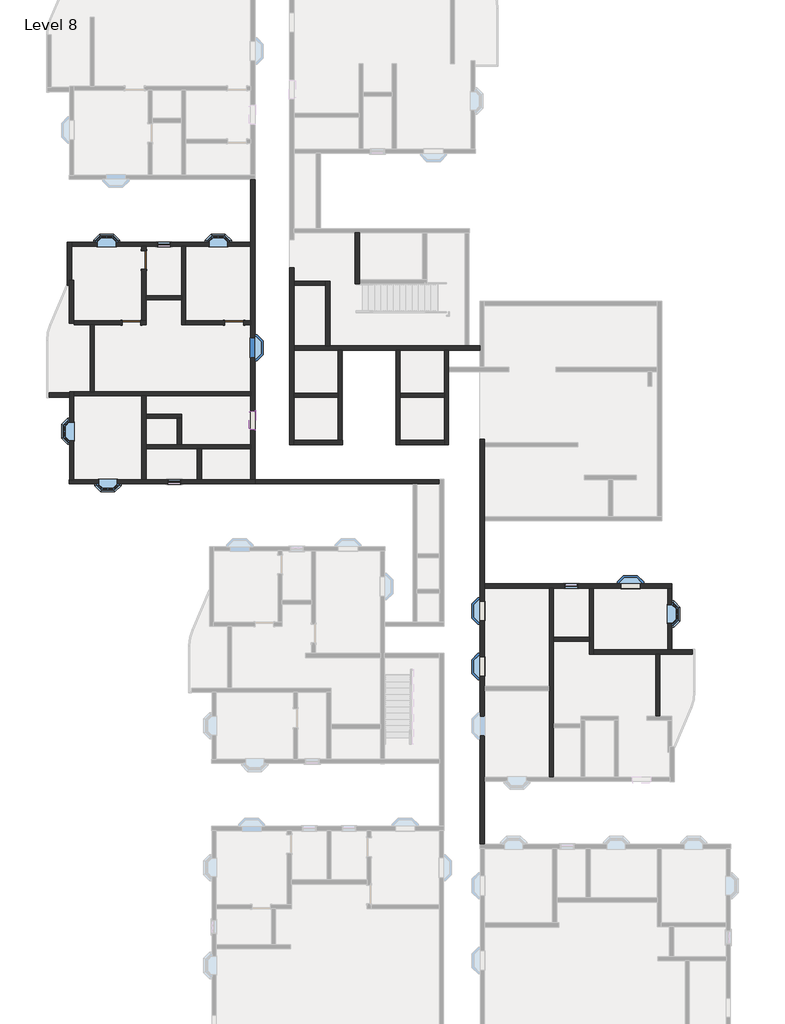
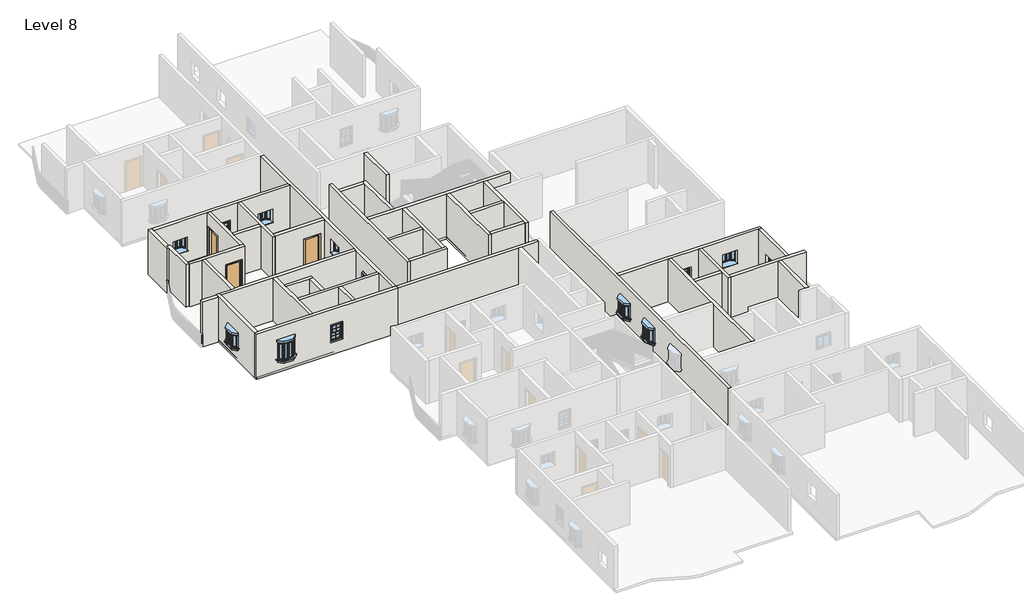
# One storey, part 3 of 14: 40 walls, 13 windows, 3 doors.
"""IFC4 building model written with IfcOpenShell, lengths in millimetres."""

from ifc_helpers import new_model, si_unit, frame, origin, place, context, project, spatial, polyline, outline, extrude, faceted_brep, transform, mapped, element, save
from components import door_54dd4da4, window_910x1210mm_154f9356, window_910x910mm_67ef725a, window_8debb0fa, windows_sgl_w_glazing_bars_910x910mm_256712d0

model = new_model("IFC4")

# Units and contexts
model_context = context("Model", 3, world=origin())
ifc_project = project(units=[si_unit("LENGTHUNIT", "METRE", prefix="MILLI")], contexts=[model_context])

# Site, building, storey
site = spatial("IfcSite", under=ifc_project)
building = spatial("IfcBuilding", under=site)
storey = spatial("IfcBuildingStorey", under=building, Name="Level 8", Elevation=21336.0)

# Doors
placement = place(None, origin())
door_shape = door_54dd4da4(model_context)
element("IfcDoor", 1, ObjectType="Single-Flush : 36\" x 84\"", at=placement, inside=storey, context=model_context, shape_type="MappedRepresentation", body=[
    mapped(door_shape, transform((-11210.3891351, 10605.7083494, 21336.0), x_axis=(1.0, 0.0, 0.0), y_axis=(0.0, 1.0, 0.0), z_axis=(0.0, 0.0, 1.0))),
])
element("IfcDoor", 2, ObjectType="Single-Flush : 36\" x 84\"", at=placement, inside=storey, context=model_context, shape_type="MappedRepresentation", body=[
    mapped(door_shape, transform((-15610.9391351, 13672.7583494, 21336.0), x_axis=(0.0, -1.0, 0.0), y_axis=(1.0, 0.0, 0.0), z_axis=(0.0, 0.0, 1.0))),
])
element("IfcDoor", 3, ObjectType="Single-Flush : 36\" x 84\"", at=placement, inside=storey, context=model_context, shape_type="MappedRepresentation", body=[
    mapped(door_shape, transform((-16220.5391351, 10605.7083494, 21336.0), x_axis=(1.0, 0.0, 0.0), y_axis=(0.0, 1.0, 0.0), z_axis=(0.0, 0.0, 1.0))),
])

# Walls
element("IfcWall", 4, ObjectType="4.5\" p", at=placement, inside=storey, context=model_context, shape_type="Brep", body=[
    faceted_brep([(-15509.3391351, 4456.3873146, 21336.0), (-13007.4391351, 4456.3873146, 21336.0), (-12804.2391351, 4456.3873146, 21336.0), (-10397.5891351, 4456.3873146, 21336.0), (-10397.5891351, 4456.3873146, 24384.0), (-12804.2391351, 4456.3873146, 24384.0), (-13007.4391351, 4456.3873146, 24384.0), (-15509.3391351, 4456.3873146, 24384.0), (-15509.3391351, 4659.5873146, 21336.0), (-15509.3391351, 4659.5873146, 24384.0), (-13985.3391351, 4659.5873146, 24384.0), (-13782.1391351, 4659.5873146, 24384.0), (-10397.5891351, 4659.5873146, 24384.0), (-10397.5891351, 4659.5873146, 21336.0), (-13782.1391351, 4659.5873146, 21336.0), (-13985.3391351, 4659.5873146, 21336.0)], [[[0, 1, 2, 3, 4, 5, 6, 7]], [[8, 9, 10, 11, 12, 13, 14, 15]], [[3, 2, 1, 0, 8, 15, 14, 13]], [[7, 6, 5, 4, 12, 11, 10, 9]], [[4, 3, 13, 12]], [[0, 7, 9, 8]]]),
])
element("IfcWall", 5, ObjectType="4.5\" p", at=placement, inside=storey, context=model_context, shape_type="SweptSolid", body=[
    extrude(outline(polyline([(-13007.4391351, 2953.9583494), (-13007.4391351, 4456.3873146), (-12804.2391351, 4456.3873146), (-12804.2391351, 2953.9583494), (-13007.4391351, 2953.9583494)])), frame((0.0, 0.0, 21336.0), z_axis=(0.0, 0.0, 1.0), x_axis=(1.0, 0.0, 0.0)), (0.0, 0.0, 1.0), 3048.0),
])
element("IfcWall", 6, ObjectType="4.5\" p", at=placement, inside=storey, context=model_context, shape_type="Brep", body=[
    faceted_brep([(-15509.3391351, 5953.2975261, 21336.0), (-13985.3391351, 5953.2975261, 21336.0), (-13782.1391351, 5953.2975261, 21336.0), (-13782.1391351, 5953.2975261, 24384.0), (-13985.3391351, 5953.2975261, 24384.0), (-15509.3391351, 5953.2975261, 24384.0), (-15509.3391351, 6156.4975261, 21336.0), (-15509.3391351, 6156.4975261, 24384.0), (-13782.1391351, 6156.4975261, 24384.0), (-13782.1391351, 6156.4975261, 21336.0)], [[[0, 1, 2, 3, 4, 5]], [[6, 7, 8, 9]], [[2, 1, 0, 6, 9]], [[5, 4, 3, 8, 7]], [[0, 5, 7, 6]], [[3, 2, 9, 8]]]),
])
element("IfcWall", 7, ObjectType="4.5\" p", at=placement, inside=storey, context=model_context, shape_type="SweptSolid", body=[
    extrude(outline(polyline([(-13985.3391351, 4659.5873146), (-13985.3391351, 5953.2975261), (-13782.1391351, 5953.2975261), (-13782.1391351, 4659.5873146), (-13985.3391351, 4659.5873146)])), frame((0.0, 0.0, 21336.0), z_axis=(0.0, 0.0, 1.0), x_axis=(1.0, 0.0, 0.0)), (0.0, 0.0, 1.0), 3048.0),
])
element("IfcWall", 8, ObjectType="4.5\" p", at=placement, inside=storey, context=model_context, shape_type="Brep", body=[
    faceted_brep([(-15712.5391351, 13215.5583494, 23469.6), (-15712.5391351, 13215.5583494, 21336.0), (-15712.5391351, 10707.3083494, 21336.0), (-15712.5391351, 10707.3083494, 24384.0), (-15712.5391351, 14333.1583494, 24384.0), (-15712.5391351, 14333.1583494, 21336.0), (-15712.5391351, 14129.9583494, 21336.0), (-15712.5391351, 14129.9583494, 23469.6), (-15509.3391351, 10707.3083494, 21336.0), (-15509.3391351, 11723.3083494, 21336.0), (-15509.3391351, 11926.5083494, 21336.0), (-15509.3391351, 13215.5583494, 21336.0), (-15509.3391351, 13215.5583494, 23469.6), (-15509.3391351, 14129.9583494, 23469.6), (-15509.3391351, 14129.9583494, 21336.0), (-15509.3391351, 14333.1583494, 21336.0), (-15509.3391351, 14333.1583494, 24384.0), (-15509.3391351, 11926.5083494, 24384.0), (-15509.3391351, 11723.3083494, 24384.0), (-15509.3391351, 10707.3083494, 24384.0)], [[[0, 1, 2, 3, 4, 5, 6, 7]], [[8, 9, 10, 11, 12, 13, 14, 15, 16, 17, 18, 19]], [[6, 5, 15, 14]], [[2, 1, 11, 10, 9, 8]], [[4, 3, 19, 18, 17, 16]], [[3, 2, 8, 19]], [[5, 4, 16, 15]], [[12, 11, 1, 0]], [[13, 12, 0, 7]], [[14, 13, 7, 6]]]),
])
element("IfcWall", 9, ObjectType="4.5\" p", at=placement, inside=storey, context=model_context, shape_type="Brep", body=[
    faceted_brep([(-13769.4391351, 14333.1583494, 21336.0), (-13769.4391351, 11926.5083494, 21336.0), (-13769.4391351, 11723.3083494, 21336.0), (-13769.4391351, 10504.1083494, 21336.0), (-13769.4391351, 10504.1083494, 24384.0), (-13769.4391351, 11723.3083494, 24384.0), (-13769.4391351, 11926.5083494, 24384.0), (-13769.4391351, 14333.1583494, 24384.0), (-13566.2391351, 14333.1583494, 21336.0), (-13566.2391351, 14333.1583494, 24384.0), (-13566.2391351, 10707.3083494, 24384.0), (-13566.2391351, 10504.1083494, 24384.0), (-13566.2391351, 10504.1083494, 21336.0), (-13566.2391351, 10707.3083494, 21336.0)], [[[0, 1, 2, 3, 4, 5, 6, 7]], [[8, 9, 10, 11, 12, 13]], [[3, 2, 1, 0, 8, 13, 12]], [[7, 6, 5, 4, 11, 10, 9]], [[0, 7, 9, 8]], [[4, 3, 12, 11]]]),
])
element("IfcWall", 10, ObjectType="4.5\" p", at=placement, inside=storey, context=model_context, shape_type="SweptSolid", body=[
    extrude(outline(polyline([(23469.6, -10753.1891351), (21336.0, -10753.1891351), (21336.0, -10397.5891351), (24384.0, -10397.5891351), (24384.0, -13566.2391351), (21336.0, -13566.2391351), (21336.0, -11667.5891351), (23469.6, -11667.5891351), (23469.6, -10753.1891351)])), frame((0.0, 10504.1083494, 0.0), z_axis=(0.0, 1.0, 0.0), x_axis=(0.0, 0.0, 1.0)), (0.0, 0.0, 1.0), 203.2),
])
element("IfcWall", 11, ObjectType="4.5\" p", at=placement, inside=storey, context=model_context, shape_type="SweptSolid", body=[
    extrude(outline(polyline([(-13769.4391351, 11723.3083494), (-15509.3391351, 11723.3083494), (-15509.3391351, 11926.5083494), (-13769.4391351, 11926.5083494), (-13769.4391351, 11723.3083494)])), frame((0.0, 0.0, 21336.0), z_axis=(0.0, 0.0, 1.0), x_axis=(1.0, 0.0, 0.0)), (0.0, 0.0, 1.0), 3048.0),
])
element("IfcWall", 12, ObjectType="4.5\" p", at=placement, inside=storey, context=model_context, shape_type="SweptSolid", body=[
    extrude(outline(polyline([(-6739.9891351, 12429.8715905), (-8289.3891351, 12429.8715905), (-8289.3891351, 12633.0715905), (-6739.9891351, 12633.0715905), (-6739.9891351, 12429.8715905)])), frame((0.0, 0.0, 21336.0), z_axis=(0.0, 0.0, 1.0), x_axis=(1.0, 0.0, 0.0)), (0.0, 0.0, 1.0), 3048.0),
])
element("IfcWall", 13, ObjectType="4.5\" p", at=placement, inside=storey, context=model_context, shape_type="SweptSolid", body=[
    extrude(outline(polyline([(-6130.3891351, 6970.2449943), (-8289.3891351, 6970.2449943), (-8289.3891351, 7173.4449943), (-6130.3891351, 7173.4449943), (-6130.3891351, 6970.2449943)])), frame((0.0, 0.0, 21336.0), z_axis=(0.0, 0.0, 1.0), x_axis=(1.0, 0.0, 0.0)), (0.0, 0.0, 1.0), 3048.0),
])
element("IfcWall", 14, ObjectType="4.5\" p", at=placement, inside=storey, context=model_context, shape_type="SweptSolid", body=[
    extrude(outline(polyline([(-948.7891351, 6970.2449943), (-3107.7891351, 6970.2449943), (-3107.7891351, 7173.4449943), (-948.7891351, 7173.4449943), (-948.7891351, 6970.2449943)])), frame((0.0, 0.0, 21336.0), z_axis=(0.0, 0.0, 1.0), x_axis=(1.0, 0.0, 0.0)), (0.0, 0.0, 1.0), 3048.0),
])
element("IfcWall", 15, ObjectType="4.5\" p", at=placement, inside=storey, context=model_context, shape_type="Brep", body=[
    faceted_brep([(-5298.5391351, 14988.9215905, 21336.0), (-5298.5391351, 12506.0715905, 21336.0), (-5298.5391351, 12506.0715905, 24384.0), (-5298.5391351, 14988.9215905, 24384.0), (-5095.3391351, 14988.9215905, 21336.0), (-5095.3391351, 14988.9215905, 24384.0), (-5095.3391351, 12709.2715905, 24384.0), (-5095.3391351, 12506.0715905, 24384.0), (-5095.3391351, 12506.0715905, 21336.0), (-5095.3391351, 12709.2715905, 21336.0)], [[[0, 1, 2, 3]], [[4, 5, 6, 7, 8, 9]], [[1, 0, 4, 9, 8]], [[3, 2, 7, 6, 5]], [[0, 3, 5, 4]], [[2, 1, 8, 7]]]),
])
element("IfcWall", 16, ObjectType="4.5\" p", at=placement, inside=storey, context=model_context, shape_type="SweptSolid", body=[
    extrude(outline(polyline([(-948.7891351, 4665.1949943), (-3107.7891351, 4665.1949943), (-3107.7891351, 4868.3949943), (-948.7891351, 4868.3949943), (-948.7891351, 4665.1949943)])), frame((0.0, 0.0, 21336.0), z_axis=(0.0, 0.0, 1.0), x_axis=(1.0, 0.0, 0.0)), (0.0, 0.0, 1.0), 3048.0),
])
element("IfcWall", 17, ObjectType="4.5\" p", at=placement, inside=storey, context=model_context, shape_type="Brep", body=[
    faceted_brep([(4184.4880523, -2336.4042694, 21336.0), (4184.4880523, -7130.6542694, 21336.0), (4184.4880523, -7333.8542694, 21336.0), (4184.4880523, -11556.6042694, 21336.0), (4184.4880523, -11556.6042694, 24384.0), (4184.4880523, -7333.8542694, 24384.0), (4184.4880523, -7130.6542694, 24384.0), (4184.4880523, -2336.4042694, 24384.0), (4387.6880523, -2336.4042694, 21336.0), (4387.6880523, -2336.4042694, 24384.0), (4387.6880523, -4736.7042694, 24384.0), (4387.6880523, -4939.9042694, 24384.0), (4387.6880523, -8959.4542694, 24384.0), (4387.6880523, -9162.6542694, 24384.0), (4387.6880523, -11556.6042694, 24384.0), (4387.6880523, -11556.6042694, 21336.0), (4387.6880523, -9162.6542694, 21336.0), (4387.6880523, -8959.4542694, 21336.0), (4387.6880523, -4939.9042694, 21336.0), (4387.6880523, -4736.7042694, 21336.0)], [[[0, 1, 2, 3, 4, 5, 6, 7]], [[8, 9, 10, 11, 12, 13, 14, 15, 16, 17, 18, 19]], [[3, 2, 1, 0, 8, 19, 18, 17, 16, 15]], [[7, 6, 5, 4, 14, 13, 12, 11, 10, 9]], [[4, 3, 15, 14]], [[0, 7, 9, 8]]]),
])
element("IfcWall", 18, ObjectType="4.5\" p", at=placement, inside=storey, context=model_context, shape_type="Brep", body=[
    faceted_brep([(803.8108649, 4915.2957306, 21336.0), (803.8108649, -14845.9042694, 21336.0), (803.8108649, -14845.9042694, 24384.0), (803.8108649, 4915.2957306, 24384.0), (803.8108649, -9516.0542694, 23446.0), (803.8108649, -9516.0542694, 22536.0), (803.8108649, -8606.0542694, 22536.0), (803.8108649, -8606.0542694, 23446.0), (803.8108649, -3909.0042694, 23446.0), (803.8108649, -3909.0042694, 22536.0), (803.8108649, -2999.0042694, 22536.0), (803.8108649, -2999.0042694, 23446.0), (803.8108649, -6620.4542694, 23446.0), (803.8108649, -6620.4542694, 22536.0), (803.8108649, -5710.4542694, 22536.0), (803.8108649, -5710.4542694, 23446.0), (1007.0108649, 4915.2957306, 21336.0), (1007.0108649, 4915.2957306, 24384.0), (1007.0108649, 4754.0949943, 24384.0), (1007.0108649, 4550.8949943, 24384.0), (1007.0108649, 1143.3957306, 24384.0), (1007.0108649, 940.1957306, 24384.0), (1007.0108649, -2133.2042694, 24384.0), (1007.0108649, -2336.4042694, 24384.0), (1007.0108649, -7130.6542694, 24384.0), (1007.0108649, -7333.8542694, 24384.0), (1007.0108649, -11556.6042694, 24384.0), (1007.0108649, -11759.8042694, 24384.0), (1007.0108649, -14845.9042694, 24384.0), (1007.0108649, -14845.9042694, 21336.0), (1007.0108649, -11759.8042694, 21336.0), (1007.0108649, -11556.6042694, 21336.0), (1007.0108649, -7333.8542694, 21336.0), (1007.0108649, -7130.6542694, 21336.0), (1007.0108649, -2336.4042694, 21336.0), (1007.0108649, -2133.2042694, 21336.0), (1007.0108649, 940.1957306, 21336.0), (1007.0108649, 1143.3957306, 21336.0), (1007.0108649, 4550.8949943, 21336.0), (1007.0108649, 4754.0949943, 21336.0), (1007.0108649, -9516.0542694, 23446.0), (1007.0108649, -8606.0542694, 23446.0), (1007.0108649, -8606.0542694, 22536.0), (1007.0108649, -9516.0542694, 22536.0), (1007.0108649, -3909.0042694, 23446.0), (1007.0108649, -2999.0042694, 23446.0), (1007.0108649, -2999.0042694, 22536.0), (1007.0108649, -3909.0042694, 22536.0), (1007.0108649, -6620.4542694, 23446.0), (1007.0108649, -5710.4542694, 23446.0), (1007.0108649, -5710.4542694, 22536.0), (1007.0108649, -6620.4542694, 22536.0)], [[[0, 1, 2, 3], [4, 5, 6, 7], [8, 9, 10, 11], [12, 13, 14, 15]], [[16, 17, 18, 19, 20, 21, 22, 23, 24, 25, 26, 27, 28, 29, 30, 31, 32, 33, 34, 35, 36, 37, 38, 39], [40, 41, 42, 43], [44, 45, 46, 47], [48, 49, 50, 51]], [[1, 0, 16, 39, 38, 37, 36, 35, 34, 33, 32, 31, 30, 29]], [[3, 2, 28, 27, 26, 25, 24, 23, 22, 21, 20, 19, 18, 17]], [[0, 3, 17, 16]], [[2, 1, 29, 28]], [[5, 4, 40, 43]], [[6, 5, 43, 42]], [[7, 6, 42, 41]], [[4, 7, 41, 40]], [[9, 8, 44, 47]], [[10, 9, 47, 46]], [[11, 10, 46, 45]], [[8, 11, 45, 44]], [[13, 12, 48, 51]], [[14, 13, 51, 50]], [[15, 14, 50, 49]], [[12, 15, 49, 48]]]),
])
element("IfcWall", 19, ObjectType="4.5\" p", at=placement, inside=storey, context=model_context, shape_type="SweptSolid", body=[
    extrude(outline(polyline([(6127.5880523, -4939.9042694), (4387.6880523, -4939.9042694), (4387.6880523, -4736.7042694), (6127.5880523, -4736.7042694), (6127.5880523, -4939.9042694)])), frame((0.0, 0.0, 21336.0), z_axis=(0.0, 0.0, 1.0), x_axis=(1.0, 0.0, 0.0)), (0.0, 0.0, 1.0), 3048.0),
])
element("IfcWall", 20, ObjectType="4.5\" p", at=placement, inside=storey, context=model_context, shape_type="Brep", body=[
    faceted_brep([(6127.5880523, -2336.4042694, 21336.0), (6127.5880523, -4736.7042694, 21336.0), (6127.5880523, -4939.9042694, 21336.0), (6127.5880523, -5555.8542694, 21336.0), (6127.5880523, -5555.8542694, 24384.0), (6127.5880523, -4939.9042694, 24384.0), (6127.5880523, -4736.7042694, 24384.0), (6127.5880523, -2336.4042694, 24384.0), (6330.7880523, -2336.4042694, 21336.0), (6330.7880523, -2336.4042694, 24384.0), (6330.7880523, -5352.6542694, 24384.0), (6330.7880523, -5555.8542694, 24384.0), (6330.7880523, -5555.8542694, 21336.0), (6330.7880523, -5352.6542694, 21336.0)], [[[0, 1, 2, 3, 4, 5, 6, 7]], [[8, 9, 10, 11, 12, 13]], [[3, 2, 1, 0, 8, 13, 12]], [[7, 6, 5, 4, 11, 10, 9]], [[0, 7, 9, 8]], [[4, 3, 12, 11]]]),
])
element("IfcWall", 21, ObjectType="4.5\" p", at=placement, inside=storey, context=model_context, shape_type="Brep", body=[
    faceted_brep([(6330.7880523, -5555.8542694, 21336.0), (9371.2322031, -5555.8542694, 21336.0), (9574.4322031, -5555.8542694, 21336.0), (11163.1380523, -5555.8542694, 21336.0), (11163.1380523, -5555.8542694, 24384.0), (9574.4322031, -5555.8542694, 24384.0), (9371.2322031, -5555.8542694, 24384.0), (6330.7880523, -5555.8542694, 24384.0), (6330.7880523, -5352.6542694, 21336.0), (6330.7880523, -5352.6542694, 24384.0), (9956.6380523, -5352.6542694, 24384.0), (10159.8380523, -5352.6542694, 24384.0), (11163.1380523, -5352.6542694, 24384.0), (11163.1380523, -5352.6542694, 21336.0), (10159.8380523, -5352.6542694, 21336.0), (9956.6380523, -5352.6542694, 21336.0)], [[[0, 1, 2, 3, 4, 5, 6, 7]], [[8, 9, 10, 11, 12, 13, 14, 15]], [[3, 2, 1, 0, 8, 15, 14, 13]], [[4, 3, 13, 12]], [[7, 6, 5, 4, 12, 11, 10, 9]], [[0, 7, 9, 8]]]),
])
element("IfcWall", 22, ObjectType="4.5\" p", at=placement, inside=storey, context=model_context, shape_type="SweptSolid", body=[
    extrude(outline(polyline([(9371.2322031, -8578.4542694), (9371.2322031, -5555.8542694), (9574.4322031, -5555.8542694), (9574.4322031, -8578.4542694), (9371.2322031, -8578.4542694)])), frame((0.0, 0.0, 21336.0), z_axis=(0.0, 0.0, 1.0), x_axis=(1.0, 0.0, 0.0)), (0.0, 0.0, 1.0), 3048.0),
])
element("IfcWall", 23, ObjectType="9\"", at=placement, inside=storey, context=model_context, shape_type="Brep", body=[
    faceted_brep([(-10181.6891351, 2953.9583494, 21336.0), (-10194.3891351, 2953.9583494, 21336.0), (-10397.5891351, 2953.9583494, 21336.0), (-12804.2391351, 2953.9583494, 21336.0), (-13007.4391351, 2953.9583494, 21336.0), (-15509.3391351, 2953.9583494, 21336.0), (-15712.5391351, 2953.9583494, 21336.0), (-19033.5891351, 2953.9583494, 21336.0), (-19236.7891351, 2953.9583494, 21336.0), (-19249.4891351, 2953.9583494, 21336.0), (-19249.4891351, 2953.9583494, 24384.0), (-19236.7891351, 2953.9583494, 24384.0), (-19033.5891351, 2953.9583494, 24384.0), (-15712.5391351, 2953.9583494, 24384.0), (-15509.3391351, 2953.9583494, 24384.0), (-13007.4391351, 2953.9583494, 24384.0), (-12804.2391351, 2953.9583494, 24384.0), (-10397.5891351, 2953.9583494, 24384.0), (-10194.3891351, 2953.9583494, 24384.0), (-10181.6891351, 2953.9583494, 24384.0), (-13794.8391351, 2953.9583494, 23317.2), (-14455.2391351, 2953.9583494, 23317.2), (-14455.2391351, 2953.9583494, 22250.4), (-13794.8391351, 2953.9583494, 22250.4), (-16918.0641351, 2953.9583494, 23446.0), (-17828.0641351, 2953.9583494, 23446.0), (-17828.0641351, 2953.9583494, 22236.0), (-16918.0641351, 2953.9583494, 22236.0), (-10181.6891351, 2750.7583494, 21336.0), (-10181.6891351, 2750.7583494, 24384.0), (-19249.4891351, 2750.7583494, 24384.0), (-19249.4891351, 2750.7583494, 21336.0), (-13794.8391351, 2750.7583494, 23317.2), (-13794.8391351, 2750.7583494, 22250.4), (-14455.2391351, 2750.7583494, 22250.4), (-14455.2391351, 2750.7583494, 23317.2), (-16918.0641351, 2750.7583494, 23446.0), (-16918.0641351, 2750.7583494, 22236.0), (-17828.0641351, 2750.7583494, 22236.0), (-17828.0641351, 2750.7583494, 23446.0)], [[[0, 1, 2, 3, 4, 5, 6, 7, 8, 9, 10, 11, 12, 13, 14, 15, 16, 17, 18, 19], [20, 21, 22, 23], [24, 25, 26, 27]], [[28, 29, 30, 31], [32, 33, 34, 35], [36, 37, 38, 39]], [[9, 8, 7, 6, 5, 4, 3, 2, 1, 0, 28, 31]], [[10, 9, 31, 30]], [[19, 18, 17, 16, 15, 14, 13, 12, 11, 10, 30, 29]], [[0, 19, 29, 28]], [[33, 32, 20, 23]], [[34, 33, 23, 22]], [[35, 34, 22, 21]], [[32, 35, 21, 20]], [[37, 36, 24, 27]], [[38, 37, 27, 26]], [[39, 38, 26, 25]], [[36, 39, 25, 24]]]),
])
element("IfcWall", 24, ObjectType="9\"", at=placement, inside=storey, context=model_context, shape_type="Brep", body=[
    faceted_brep([(-19033.5891351, 2953.9583494, 21336.0), (-19033.5891351, 7037.0083494, 21336.0), (-19033.5891351, 7240.2083494, 21336.0), (-19033.5891351, 7240.2083494, 24384.0), (-19033.5891351, 7037.0083494, 24384.0), (-19033.5891351, 2953.9583494, 24384.0), (-19033.5891351, 4854.8083494, 23160.4), (-19033.5891351, 5764.8083494, 23160.4), (-19033.5891351, 5764.8083494, 22250.4), (-19033.5891351, 4854.8083494, 22250.4), (-19236.7891351, 2953.9583494, 21336.0), (-19236.7891351, 2953.9583494, 24384.0), (-19236.7891351, 7240.2083494, 24384.0), (-19236.7891351, 7240.2083494, 21336.0), (-19236.7891351, 4854.8083494, 23160.4), (-19236.7891351, 4854.8083494, 22250.4), (-19236.7891351, 5764.8083494, 22250.4), (-19236.7891351, 5764.8083494, 23160.4)], [[[0, 1, 2, 3, 4, 5], [6, 7, 8, 9]], [[10, 11, 12, 13], [14, 15, 16, 17]], [[2, 1, 0, 10, 13]], [[5, 4, 3, 12, 11]], [[0, 5, 11, 10]], [[3, 2, 13, 12]], [[15, 14, 6, 9]], [[16, 15, 9, 8]], [[17, 16, 8, 7]], [[14, 17, 7, 6]]]),
])
element("IfcWall", 25, ObjectType="9\"", at=placement, inside=storey, context=model_context, shape_type="Brep", body=[
    faceted_brep([(-10194.3891351, 2953.9583494, 21336.0), (-10194.3891351, 17597.0583494, 21336.0), (-10194.3891351, 17597.0583494, 24384.0), (-10194.3891351, 2953.9583494, 24384.0), (-10194.3891351, 9841.5083494, 23446.0), (-10194.3891351, 9841.5083494, 22536.0), (-10194.3891351, 8931.5083494, 22536.0), (-10194.3891351, 8931.5083494, 23446.0), (-10194.3891351, 5393.297832, 23446.0), (-10194.3891351, 6303.297832, 23446.0), (-10194.3891351, 6303.297832, 22536.0), (-10194.3891351, 5393.297832, 22536.0), (-10397.5891351, 2953.9583494, 21336.0), (-10397.5891351, 2953.9583494, 24384.0), (-10397.5891351, 4456.3873146, 24384.0), (-10397.5891351, 4659.5873146, 24384.0), (-10397.5891351, 7037.0083494, 24384.0), (-10397.5891351, 7240.2083494, 24384.0), (-10397.5891351, 10504.1083494, 24384.0), (-10397.5891351, 10707.3083494, 24384.0), (-10397.5891351, 14333.1583494, 24384.0), (-10397.5891351, 14536.3583494, 24384.0), (-10397.5891351, 17597.0583494, 24384.0), (-10397.5891351, 17597.0583494, 21336.0), (-10397.5891351, 14536.3583494, 21336.0), (-10397.5891351, 14333.1583494, 21336.0), (-10397.5891351, 10707.3083494, 21336.0), (-10397.5891351, 10504.1083494, 21336.0), (-10397.5891351, 7240.2083494, 21336.0), (-10397.5891351, 7037.0083494, 21336.0), (-10397.5891351, 4659.5873146, 21336.0), (-10397.5891351, 4456.3873146, 21336.0), (-10397.5891351, 9841.5083494, 23446.0), (-10397.5891351, 8931.5083494, 23446.0), (-10397.5891351, 8931.5083494, 22536.0), (-10397.5891351, 9841.5083494, 22536.0), (-10397.5891351, 5393.297832, 23446.0), (-10397.5891351, 5393.297832, 22536.0), (-10397.5891351, 6303.297832, 22536.0), (-10397.5891351, 6303.297832, 23446.0)], [[[0, 1, 2, 3], [4, 5, 6, 7], [8, 9, 10, 11]], [[12, 13, 14, 15, 16, 17, 18, 19, 20, 21, 22, 23, 24, 25, 26, 27, 28, 29, 30, 31], [32, 33, 34, 35], [36, 37, 38, 39]], [[1, 0, 12, 31, 30, 29, 28, 27, 26, 25, 24, 23]], [[2, 1, 23, 22]], [[3, 2, 22, 21, 20, 19, 18, 17, 16, 15, 14, 13]], [[0, 3, 13, 12]], [[5, 4, 32, 35]], [[6, 5, 35, 34]], [[7, 6, 34, 33]], [[4, 7, 33, 32]], [[37, 36, 8, 11]], [[38, 37, 11, 10]], [[39, 38, 10, 9]], [[36, 39, 9, 8]]]),
])
element("IfcWall", 26, ObjectType="9\"", at=placement, inside=storey, context=model_context, shape_type="SweptSolid", body=[
    extrude(outline(polyline([(-19249.4891351, 6979.8583494), (-20240.0891351, 6979.8583494), (-20240.0891351, 7183.0583494), (-19249.4891351, 7183.0583494), (-19249.4891351, 6979.8583494)])), frame((0.0, 0.0, 21336.0), z_axis=(0.0, 0.0, 1.0), x_axis=(1.0, 0.0, 0.0)), (0.0, 0.0, 1.0), 3048.0),
])
element("IfcWall", 27, ObjectType="9\"", at=placement, inside=storey, context=model_context, shape_type="Brep", body=[
    faceted_brep([(-19147.8891351, 12435.1858981, 21336.0), (-19147.8891351, 14333.1583494, 21336.0), (-19147.8891351, 14536.3583494, 21336.0), (-19147.8891351, 14549.0583494, 21336.0), (-19147.8891351, 14549.0583494, 24384.0), (-19147.8891351, 14536.3583494, 24384.0), (-19147.8891351, 14333.1583494, 24384.0), (-19147.8891351, 12435.1858981, 24384.0), (-19351.0891351, 12435.1858981, 21336.0), (-19351.0891351, 12435.1858981, 24384.0), (-19351.0891351, 14549.0583494, 24384.0), (-19351.0891351, 14549.0583494, 21336.0)], [[[0, 1, 2, 3, 4, 5, 6, 7]], [[8, 9, 10, 11]], [[3, 2, 1, 0, 8, 11]], [[4, 3, 11, 10]], [[7, 6, 5, 4, 10, 9]], [[0, 7, 9, 8]]]),
])
element("IfcWall", 28, ObjectType="9\"", at=placement, inside=storey, context=model_context, shape_type="Brep", body=[
    faceted_brep([(-19147.8891351, 14333.1583494, 21336.0), (-15712.5391351, 14333.1583494, 21336.0), (-15509.3391351, 14333.1583494, 21336.0), (-13769.4391351, 14333.1583494, 21336.0), (-13566.2391351, 14333.1583494, 21336.0), (-10397.5891351, 14333.1583494, 21336.0), (-10397.5891351, 14333.1583494, 24384.0), (-13566.2391351, 14333.1583494, 24384.0), (-13769.4391351, 14333.1583494, 24384.0), (-15509.3391351, 14333.1583494, 24384.0), (-15712.5391351, 14333.1583494, 24384.0), (-19147.8891351, 14333.1583494, 24384.0), (-17885.2141351, 14333.1583494, 23160.4), (-16975.2141351, 14333.1583494, 23160.4), (-16975.2141351, 14333.1583494, 22250.4), (-17885.2141351, 14333.1583494, 22250.4), (-12436.9141351, 14333.1583494, 23160.4), (-11526.9141351, 14333.1583494, 23160.4), (-11526.9141351, 14333.1583494, 22250.4), (-12436.9141351, 14333.1583494, 22250.4), (-14309.1891351, 14333.1583494, 23317.2), (-14309.1891351, 14333.1583494, 22250.4), (-14969.5891351, 14333.1583494, 22250.4), (-14969.5891351, 14333.1583494, 23317.2), (-19147.8891351, 14536.3583494, 21336.0), (-19147.8891351, 14536.3583494, 24384.0), (-10397.5891351, 14536.3583494, 24384.0), (-10397.5891351, 14536.3583494, 21336.0), (-17885.2141351, 14536.3583494, 23160.4), (-17885.2141351, 14536.3583494, 22250.4), (-16975.2141351, 14536.3583494, 22250.4), (-16975.2141351, 14536.3583494, 23160.4), (-12436.9141351, 14536.3583494, 23160.4), (-12436.9141351, 14536.3583494, 22250.4), (-11526.9141351, 14536.3583494, 22250.4), (-11526.9141351, 14536.3583494, 23160.4), (-14309.1891351, 14536.3583494, 23317.2), (-14969.5891351, 14536.3583494, 23317.2), (-14969.5891351, 14536.3583494, 22250.4), (-14309.1891351, 14536.3583494, 22250.4)], [[[0, 1, 2, 3, 4, 5, 6, 7, 8, 9, 10, 11], [12, 13, 14, 15], [16, 17, 18, 19], [20, 21, 22, 23]], [[24, 25, 26, 27], [28, 29, 30, 31], [32, 33, 34, 35], [36, 37, 38, 39]], [[5, 4, 3, 2, 1, 0, 24, 27]], [[11, 10, 9, 8, 7, 6, 26, 25]], [[6, 5, 27, 26]], [[0, 11, 25, 24]], [[29, 28, 12, 15]], [[30, 29, 15, 14]], [[31, 30, 14, 13]], [[28, 31, 13, 12]], [[33, 32, 16, 19]], [[34, 33, 19, 18]], [[35, 34, 18, 17]], [[32, 35, 17, 16]], [[21, 20, 36, 39]], [[22, 21, 39, 38]], [[23, 22, 38, 37]], [[20, 23, 37, 36]]]),
])
element("IfcWall", 29, ObjectType="9\"", at=placement, inside=storey, context=model_context, shape_type="SweptSolid", body=[
    extrude(outline(polyline([(-19249.4891351, 10585.5474528), (-19249.4891351, 12672.4473407), (-19046.2891351, 12672.4473407), (-19046.2891351, 10585.5474528), (-19249.4891351, 10585.5474528)])), frame((0.0, 0.0, 21336.0), z_axis=(0.0, 0.0, 1.0), x_axis=(1.0, 0.0, 0.0)), (0.0, 0.0, 1.0), 3048.0),
])
element("IfcWall", 30, ObjectType="9\" w", at=placement, inside=storey, context=model_context, shape_type="Brep", body=[
    faceted_brep([(-1177.3891351, 2953.9583494, 21336.0), (-10181.6891351, 2953.9583494, 21336.0), (-10181.6891351, 2953.9583494, 24384.0), (-1177.3891351, 2953.9583494, 24384.0), (-1177.3891351, 2750.7583494, 21336.0), (-1177.3891351, 2750.7583494, 24384.0), (-2269.5891351, 2750.7583494, 24384.0), (-2472.7891351, 2750.7583494, 24384.0), (-10181.6891351, 2750.7583494, 24384.0), (-10181.6891351, 2750.7583494, 21336.0), (-2472.7891351, 2750.7583494, 21336.0), (-2269.5891351, 2750.7583494, 21336.0)], [[[0, 1, 2, 3]], [[4, 5, 6, 7, 8, 9, 10, 11]], [[1, 0, 4, 11, 10, 9]], [[2, 1, 9, 8]], [[3, 2, 8, 7, 6, 5]], [[0, 3, 5, 4]]]),
])
element("IfcWall", 31, ObjectType="9\" w", at=placement, inside=storey, context=model_context, shape_type="Brep", body=[
    faceted_brep([(-15763.3391351, 10504.1083494, 23469.6), (-15763.3391351, 10504.1083494, 21336.0), (-15509.3391351, 10504.1083494, 21336.0), (-15509.3391351, 10504.1083494, 24384.0), (-18042.9891351, 10504.1083494, 24384.0), (-18246.1891351, 10504.1083494, 24384.0), (-19027.2391351, 10504.1083494, 24384.0), (-19027.2391351, 10504.1083494, 21336.0), (-18246.1891351, 10504.1083494, 21336.0), (-18042.9891351, 10504.1083494, 21336.0), (-16677.7391351, 10504.1083494, 21336.0), (-16677.7391351, 10504.1083494, 23469.6), (-15509.3391351, 10707.3083494, 21336.0), (-15712.5391351, 10707.3083494, 21336.0), (-15763.3391351, 10707.3083494, 21336.0), (-15763.3391351, 10707.3083494, 23469.6), (-16677.7391351, 10707.3083494, 23469.6), (-16677.7391351, 10707.3083494, 21336.0), (-19027.2391351, 10707.3083494, 21336.0), (-19027.2391351, 10707.3083494, 24384.0), (-15712.5391351, 10707.3083494, 24384.0), (-15509.3391351, 10707.3083494, 24384.0)], [[[0, 1, 2, 3, 4, 5, 6, 7, 8, 9, 10, 11]], [[12, 13, 14, 15, 16, 17, 18, 19, 20, 21]], [[2, 1, 14, 13, 12]], [[10, 9, 8, 7, 18, 17]], [[6, 5, 4, 3, 21, 20, 19]], [[7, 6, 19, 18]], [[3, 2, 12, 21]], [[15, 14, 1, 0]], [[16, 15, 0, 11]], [[17, 16, 11, 10]]]),
])
element("IfcWall", 32, ObjectType="9\" w", at=placement, inside=storey, context=model_context, shape_type="SweptSolid", body=[
    extrude(outline(polyline([(-18246.1891351, 7240.2083494), (-18246.1891351, 10504.1083494), (-18042.9891351, 10504.1083494), (-18042.9891351, 7240.2083494), (-18246.1891351, 7240.2083494)])), frame((0.0, 0.0, 21336.0), z_axis=(0.0, 0.0, 1.0), x_axis=(1.0, 0.0, 0.0)), (0.0, 0.0, 1.0), 3048.0),
])
element("IfcWall", 33, ObjectType="9\" w", at=placement, inside=storey, context=model_context, shape_type="Brep", body=[
    faceted_brep([(-19033.5891351, 7037.0083494, 21336.0), (-15712.5391351, 7037.0083494, 21336.0), (-15509.3391351, 7037.0083494, 21336.0), (-10397.5891351, 7037.0083494, 21336.0), (-10397.5891351, 7037.0083494, 24384.0), (-15509.3391351, 7037.0083494, 24384.0), (-15712.5391351, 7037.0083494, 24384.0), (-19033.5891351, 7037.0083494, 24384.0), (-19033.5891351, 7240.2083494, 21336.0), (-19033.5891351, 7240.2083494, 24384.0), (-18246.1891351, 7240.2083494, 24384.0), (-18042.9891351, 7240.2083494, 24384.0), (-10397.5891351, 7240.2083494, 24384.0), (-10397.5891351, 7240.2083494, 21336.0), (-18042.9891351, 7240.2083494, 21336.0), (-18246.1891351, 7240.2083494, 21336.0)], [[[0, 1, 2, 3, 4, 5, 6, 7]], [[8, 9, 10, 11, 12, 13, 14, 15]], [[3, 2, 1, 0, 8, 15, 14, 13]], [[7, 6, 5, 4, 12, 11, 10, 9]], [[0, 7, 9, 8]], [[4, 3, 13, 12]]]),
])
element("IfcWall", 34, ObjectType="9\" w", at=placement, inside=storey, context=model_context, shape_type="Brep", body=[
    faceted_brep([(-15712.5391351, 7037.0083494, 21336.0), (-15712.5391351, 2953.9583494, 21336.0), (-15712.5391351, 2953.9583494, 24384.0), (-15712.5391351, 7037.0083494, 24384.0), (-15509.3391351, 7037.0083494, 21336.0), (-15509.3391351, 7037.0083494, 24384.0), (-15509.3391351, 6156.4975261, 24384.0), (-15509.3391351, 5953.2975261, 24384.0), (-15509.3391351, 4659.5873146, 24384.0), (-15509.3391351, 4456.3873146, 24384.0), (-15509.3391351, 2953.9583494, 24384.0), (-15509.3391351, 2953.9583494, 21336.0), (-15509.3391351, 4456.3873146, 21336.0), (-15509.3391351, 4659.5873146, 21336.0), (-15509.3391351, 5953.2975261, 21336.0), (-15509.3391351, 6156.4975261, 21336.0)], [[[0, 1, 2, 3]], [[4, 5, 6, 7, 8, 9, 10, 11, 12, 13, 14, 15]], [[1, 0, 4, 15, 14, 13, 12, 11]], [[3, 2, 10, 9, 8, 7, 6, 5]], [[2, 1, 11, 10]], [[0, 3, 5, 4]]]),
])
element("IfcWall", 35, ObjectType="9\" w", at=placement, inside=storey, context=model_context, shape_type="Brep", body=[
    faceted_brep([(-8492.5891351, 13295.1410318, 21336.0), (-8492.5891351, 4652.4949943, 21336.0), (-8492.5891351, 4652.4949943, 24384.0), (-8492.5891351, 13295.1410318, 24384.0), (-8289.3891351, 13295.1410318, 21336.0), (-8289.3891351, 13295.1410318, 24384.0), (-8289.3891351, 12633.0715905, 24384.0), (-8289.3891351, 12429.8715905, 24384.0), (-8289.3891351, 9478.4949943, 24384.0), (-8289.3891351, 9275.2949943, 24384.0), (-8289.3891351, 7173.4449943, 24384.0), (-8289.3891351, 6970.2449943, 24384.0), (-8289.3891351, 4868.3949943, 24384.0), (-8289.3891351, 4665.1949943, 24384.0), (-8289.3891351, 4652.4949943, 24384.0), (-8289.3891351, 4652.4949943, 21336.0), (-8289.3891351, 4665.1949943, 21336.0), (-8289.3891351, 4868.3949943, 21336.0), (-8289.3891351, 6970.2449943, 21336.0), (-8289.3891351, 7173.4449943, 21336.0), (-8289.3891351, 9275.2949943, 21336.0), (-8289.3891351, 9478.4949943, 21336.0), (-8289.3891351, 12429.8715905, 21336.0), (-8289.3891351, 12633.0715905, 21336.0)], [[[0, 1, 2, 3]], [[4, 5, 6, 7, 8, 9, 10, 11, 12, 13, 14, 15, 16, 17, 18, 19, 20, 21, 22, 23]], [[1, 0, 4, 23, 22, 21, 20, 19, 18, 17, 16, 15]], [[2, 1, 15, 14]], [[3, 2, 14, 13, 12, 11, 10, 9, 8, 7, 6, 5]], [[0, 3, 5, 4]]]),
])
element("IfcWall", 36, ObjectType="9\" w", at=placement, inside=storey, context=model_context, shape_type="Brep", body=[
    faceted_brep([(-8289.3891351, 4665.1949943, 21336.0), (-5914.4891351, 4665.1949943, 21336.0), (-5914.4891351, 4665.1949943, 24384.0), (-8289.3891351, 4665.1949943, 24384.0), (-8289.3891351, 4868.3949943, 21336.0), (-8289.3891351, 4868.3949943, 24384.0), (-6130.3891351, 4868.3949943, 24384.0), (-5927.1891351, 4868.3949943, 24384.0), (-5914.4891351, 4868.3949943, 24384.0), (-5914.4891351, 4868.3949943, 21336.0), (-5927.1891351, 4868.3949943, 21336.0), (-6130.3891351, 4868.3949943, 21336.0)], [[[0, 1, 2, 3]], [[4, 5, 6, 7, 8, 9, 10, 11]], [[1, 0, 4, 11, 10, 9]], [[2, 1, 9, 8]], [[3, 2, 8, 7, 6, 5]], [[0, 3, 5, 4]]]),
])
element("IfcWall", 37, ObjectType="9\" w", at=placement, inside=storey, context=model_context, shape_type="Brep", body=[
    faceted_brep([(-5927.1891351, 4868.3949943, 21336.0), (-5927.1891351, 9275.2949943, 21336.0), (-5927.1891351, 9275.2949943, 24384.0), (-5927.1891351, 4868.3949943, 24384.0), (-6130.3891351, 4868.3949943, 21336.0), (-6130.3891351, 4868.3949943, 24384.0), (-6130.3891351, 6970.2449943, 24384.0), (-6130.3891351, 7173.4449943, 24384.0), (-6130.3891351, 9275.2949943, 24384.0), (-6130.3891351, 9275.2949943, 21336.0), (-6130.3891351, 7173.4449943, 21336.0), (-6130.3891351, 6970.2449943, 21336.0)], [[[0, 1, 2, 3]], [[4, 5, 6, 7, 8, 9, 10, 11]], [[1, 0, 4, 11, 10, 9]], [[3, 2, 8, 7, 6, 5]], [[0, 3, 5, 4]], [[2, 1, 9, 8]]]),
])
element("IfcWall", 38, ObjectType="9\" w", at=placement, inside=storey, context=model_context, shape_type="Brep", body=[
    faceted_brep([(-8289.3891351, 9275.2949943, 21336.0), (-6130.3891351, 9275.2949943, 21336.0), (-5927.1891351, 9275.2949943, 21336.0), (-3310.9891351, 9275.2949943, 21336.0), (-3107.7891351, 9275.2949943, 21336.0), (-948.7891351, 9275.2949943, 21336.0), (-745.5891351, 9275.2949943, 21336.0), (793.5880523, 9275.2949943, 21336.0), (793.5880523, 9275.2949943, 24384.0), (-745.5891351, 9275.2949943, 24384.0), (-948.7891351, 9275.2949943, 24384.0), (-3107.7891351, 9275.2949943, 24384.0), (-3310.9891351, 9275.2949943, 24384.0), (-5927.1891351, 9275.2949943, 24384.0), (-6130.3891351, 9275.2949943, 24384.0), (-8289.3891351, 9275.2949943, 24384.0), (-8289.3891351, 9478.4949943, 21336.0), (-8289.3891351, 9478.4949943, 24384.0), (-6739.9891351, 9478.4949943, 24384.0), (-6536.7891351, 9478.4949943, 24384.0), (54.5108649, 9478.4949943, 24384.0), (257.7108649, 9478.4949943, 24384.0), (793.5880523, 9478.4949943, 24384.0), (793.5880523, 9478.4949943, 21336.0), (257.7108649, 9478.4949943, 21336.0), (54.5108649, 9478.4949943, 21336.0), (-6536.7891351, 9478.4949943, 21336.0), (-6739.9891351, 9478.4949943, 21336.0)], [[[0, 1, 2, 3, 4, 5, 6, 7, 8, 9, 10, 11, 12, 13, 14, 15]], [[16, 17, 18, 19, 20, 21, 22, 23, 24, 25, 26, 27]], [[7, 6, 5, 4, 3, 2, 1, 0, 16, 27, 26, 25, 24, 23]], [[15, 14, 13, 12, 11, 10, 9, 8, 22, 21, 20, 19, 18, 17]], [[0, 15, 17, 16]], [[8, 7, 23, 22]]]),
])
element("IfcWall", 39, ObjectType="9\" w", at=placement, inside=storey, context=model_context, shape_type="Brep", body=[
    faceted_brep([(-3310.9891351, 9275.2949943, 21336.0), (-3310.9891351, 4652.4949943, 21336.0), (-3310.9891351, 4652.4949943, 24384.0), (-3310.9891351, 9275.2949943, 24384.0), (-3107.7891351, 9275.2949943, 21336.0), (-3107.7891351, 9275.2949943, 24384.0), (-3107.7891351, 7173.4449943, 24384.0), (-3107.7891351, 6970.2449943, 24384.0), (-3107.7891351, 4868.3949943, 24384.0), (-3107.7891351, 4665.1949943, 24384.0), (-3107.7891351, 4652.4949943, 24384.0), (-3107.7891351, 4652.4949943, 21336.0), (-3107.7891351, 4665.1949943, 21336.0), (-3107.7891351, 4868.3949943, 21336.0), (-3107.7891351, 6970.2449943, 21336.0), (-3107.7891351, 7173.4449943, 21336.0)], [[[0, 1, 2, 3]], [[4, 5, 6, 7, 8, 9, 10, 11, 12, 13, 14, 15]], [[1, 0, 4, 15, 14, 13, 12, 11]], [[2, 1, 11, 10]], [[3, 2, 10, 9, 8, 7, 6, 5]], [[0, 3, 5, 4]]]),
])
element("IfcWall", 40, ObjectType="9\" w", at=placement, inside=storey, context=model_context, shape_type="Brep", body=[
    faceted_brep([(-745.5891351, 4652.4949943, 21336.0), (-745.5891351, 8223.6457306, 21336.0), (-745.5891351, 8426.8457306, 21336.0), (-745.5891351, 9275.2949943, 21336.0), (-745.5891351, 9275.2949943, 24384.0), (-745.5891351, 8426.8457306, 24384.0), (-745.5891351, 8223.6457306, 24384.0), (-745.5891351, 4652.4949943, 24384.0), (-948.7891351, 4652.4949943, 21336.0), (-948.7891351, 4652.4949943, 24384.0), (-948.7891351, 4665.1949943, 24384.0), (-948.7891351, 4868.3949943, 24384.0), (-948.7891351, 6970.2449943, 24384.0), (-948.7891351, 7173.4449943, 24384.0), (-948.7891351, 9275.2949943, 24384.0), (-948.7891351, 9275.2949943, 21336.0), (-948.7891351, 7173.4449943, 21336.0), (-948.7891351, 6970.2449943, 21336.0), (-948.7891351, 4868.3949943, 21336.0), (-948.7891351, 4665.1949943, 21336.0)], [[[0, 1, 2, 3, 4, 5, 6, 7]], [[8, 9, 10, 11, 12, 13, 14, 15, 16, 17, 18, 19]], [[3, 2, 1, 0, 8, 19, 18, 17, 16, 15]], [[7, 6, 5, 4, 14, 13, 12, 11, 10, 9]], [[0, 7, 9, 8]], [[4, 3, 15, 14]]]),
])
element("IfcWall", 41, ObjectType="9\" w", at=placement, inside=storey, context=model_context, shape_type="Brep", body=[
    faceted_brep([(-6536.7891351, 9478.4949943, 21336.0), (-6536.7891351, 12633.0715905, 21336.0), (-6536.7891351, 12633.0715905, 24384.0), (-6536.7891351, 9478.4949943, 24384.0), (-6739.9891351, 9478.4949943, 21336.0), (-6739.9891351, 9478.4949943, 24384.0), (-6739.9891351, 12429.8715905, 24384.0), (-6739.9891351, 12633.0715905, 24384.0), (-6739.9891351, 12633.0715905, 21336.0), (-6739.9891351, 12429.8715905, 21336.0)], [[[0, 1, 2, 3]], [[4, 5, 6, 7, 8, 9]], [[1, 0, 4, 9, 8]], [[3, 2, 7, 6, 5]], [[0, 3, 5, 4]], [[2, 1, 8, 7]]]),
])
element("IfcWall", 42, ObjectType="9\" w", at=placement, inside=storey, context=model_context, shape_type="Brep", body=[
    faceted_brep([(1007.0108649, -2336.4042694, 21336.0), (4184.4880523, -2336.4042694, 21336.0), (4387.6880523, -2336.4042694, 21336.0), (6127.5880523, -2336.4042694, 21336.0), (6330.7880523, -2336.4042694, 21336.0), (9956.6380523, -2336.4042694, 21336.0), (10159.8380523, -2336.4042694, 21336.0), (10172.5380523, -2336.4042694, 21336.0), (10172.5380523, -2336.4042694, 24384.0), (10159.8380523, -2336.4042694, 24384.0), (9956.6380523, -2336.4042694, 24384.0), (6330.7880523, -2336.4042694, 24384.0), (6127.5880523, -2336.4042694, 24384.0), (4387.6880523, -2336.4042694, 24384.0), (4184.4880523, -2336.4042694, 24384.0), (1007.0108649, -2336.4042694, 24384.0), (7688.7130523, -2336.4042694, 23446.0), (8598.7130523, -2336.4042694, 23446.0), (8598.7130523, -2336.4042694, 22536.0), (7688.7130523, -2336.4042694, 22536.0), (4927.4380523, -2336.4042694, 23317.2), (5587.8380523, -2336.4042694, 23317.2), (5587.8380523, -2336.4042694, 22250.4), (4927.4380523, -2336.4042694, 22250.4), (1007.0108649, -2133.2042694, 21336.0), (1007.0108649, -2133.2042694, 24384.0), (10172.5380523, -2133.2042694, 24384.0), (10172.5380523, -2133.2042694, 21336.0), (7688.7130523, -2133.2042694, 23446.0), (7688.7130523, -2133.2042694, 22536.0), (8598.7130523, -2133.2042694, 22536.0), (8598.7130523, -2133.2042694, 23446.0), (4927.4380523, -2133.2042694, 23317.2), (4927.4380523, -2133.2042694, 22250.4), (5587.8380523, -2133.2042694, 22250.4), (5587.8380523, -2133.2042694, 23317.2)], [[[0, 1, 2, 3, 4, 5, 6, 7, 8, 9, 10, 11, 12, 13, 14, 15], [16, 17, 18, 19], [20, 21, 22, 23]], [[24, 25, 26, 27], [28, 29, 30, 31], [32, 33, 34, 35]], [[7, 6, 5, 4, 3, 2, 1, 0, 24, 27]], [[8, 7, 27, 26]], [[15, 14, 13, 12, 11, 10, 9, 8, 26, 25]], [[0, 15, 25, 24]], [[29, 28, 16, 19]], [[30, 29, 19, 18]], [[31, 30, 18, 17]], [[28, 31, 17, 16]], [[33, 32, 20, 23]], [[34, 33, 23, 22]], [[35, 34, 22, 21]], [[32, 35, 21, 20]]]),
])
element("IfcWall", 43, ObjectType="9\" w", at=placement, inside=storey, context=model_context, shape_type="SweptSolid", body=[
    extrude(outline(polyline([(-2336.4042694, 21336.0), (-5352.6542694, 21336.0), (-5352.6542694, 24384.0), (-2336.4042694, 24384.0), (-2336.4042694, 21336.0)]), holes=[polyline([(-3151.4042694, 23160.4), (-4061.4042694, 23160.4), (-4061.4042694, 22250.4), (-3151.4042694, 22250.4), (-3151.4042694, 23160.4)])]), frame((9956.6380523, 0.0, 0.0), z_axis=(1.0, 0.0, 0.0), x_axis=(0.0, 1.0, 0.0)), (0.0, 0.0, 1.0), 203.2),
])

# Windows
window_910x1210mm_shape = window_910x1210mm_154f9356(model_context)
element("IfcWindow", 44, ObjectType="910x1210mm", at=placement, inside=storey, context=model_context, shape_type="MappedRepresentation", body=[
    mapped(window_910x1210mm_shape, transform((-17943.0641351, 2860.8149172, 21336.0), x_axis=(-1.0, 0.0, 0.0), y_axis=(0.0, -1.0, 0.0), z_axis=(0.0, 0.0, 1.0))),
])
window_910x910mm_shape = window_910x910mm_67ef725a(model_context)
element("IfcWindow", 45, ObjectType="910x910mm", at=placement, inside=storey, context=model_context, shape_type="MappedRepresentation", body=[
    mapped(window_910x910mm_shape, transform((8713.7130523, -2243.2608372, 21336.0), x_axis=(1.0, 0.0, 0.0), y_axis=(0.0, 1.0, 0.0), z_axis=(0.0, 0.0, 1.0))),
])
element("IfcWindow", 46, ObjectType="910x910mm", at=placement, inside=storey, context=model_context, shape_type="MappedRepresentation", body=[
    mapped(window_910x910mm_shape, transform((10049.7814845, -4176.4042694, 21050.4), x_axis=(0.0, -1.0, 0.0), y_axis=(1.0, 0.0, 0.0), z_axis=(0.0, 0.0, 1.0))),
])
element("IfcWindow", 47, ObjectType="910x910mm", at=placement, inside=storey, context=model_context, shape_type="MappedRepresentation", body=[
    mapped(window_910x910mm_shape, transform((-16860.2141351, 14426.3017816, 21050.4), x_axis=(1.0, 0.0, 0.0), y_axis=(0.0, 1.0, 0.0), z_axis=(0.0, 0.0, 1.0))),
])
element("IfcWindow", 48, ObjectType="910x910mm", at=placement, inside=storey, context=model_context, shape_type="MappedRepresentation", body=[
    mapped(window_910x910mm_shape, transform((-11411.9141351, 14426.3017816, 21050.4), x_axis=(1.0, 0.0, 0.0), y_axis=(0.0, 1.0, 0.0), z_axis=(0.0, 0.0, 1.0))),
])
element("IfcWindow", 49, ObjectType="910x910mm", at=placement, inside=storey, context=model_context, shape_type="MappedRepresentation", body=[
    mapped(window_910x910mm_shape, transform((-10304.445703, 8816.5083494, 21336.0), x_axis=(0.0, -1.0, 0.0), y_axis=(1.0, 0.0, 0.0), z_axis=(0.0, 0.0, 1.0))),
])
element("IfcWindow", 50, ObjectType="910x910mm", at=placement, inside=storey, context=model_context, shape_type="MappedRepresentation", body=[
    mapped(window_910x910mm_shape, transform((-19126.7325673, 5879.8083494, 21050.4), x_axis=(0.0, 1.0, 0.0), y_axis=(-1.0, 0.0, 0.0), z_axis=(0.0, 0.0, 1.0))),
])
element("IfcWindow", 51, ObjectType="910x910mm", at=placement, inside=storey, context=model_context, shape_type="MappedRepresentation", body=[
    mapped(window_910x910mm_shape, transform((913.8674327, -2884.0042694, 21336.0), x_axis=(0.0, 1.0, 0.0), y_axis=(-1.0, 0.0, 0.0), z_axis=(0.0, 0.0, 1.0))),
])
element("IfcWindow", 52, ObjectType="910x910mm", at=placement, inside=storey, context=model_context, shape_type="MappedRepresentation", body=[
    mapped(window_910x910mm_shape, transform((913.8674327, -5595.4542694, 21336.0), x_axis=(0.0, 1.0, 0.0), y_axis=(-1.0, 0.0, 0.0), z_axis=(0.0, 0.0, 1.0))),
])
window_shape = window_8debb0fa(model_context)
element("IfcWindow", 53, ObjectType="Window-Double-Hung : 26\" x 42\"", at=placement, inside=storey, context=model_context, shape_type="MappedRepresentation", body=[
    mapped(window_shape, transform((5257.6380523, -2234.8042694, 21336.0), x_axis=(1.0, 0.0, 0.0), y_axis=(0.0, 1.0, 0.0), z_axis=(0.0, 0.0, 1.0))),
])
element("IfcWindow", 54, ObjectType="Window-Double-Hung : 26\" x 42\"", at=placement, inside=storey, context=model_context, shape_type="MappedRepresentation", body=[
    mapped(window_shape, transform((-14639.3891351, 14434.7583494, 21336.0), x_axis=(-1.0, 0.0, 0.0), y_axis=(0.0, -1.0, 0.0), z_axis=(0.0, 0.0, 1.0))),
])
element("IfcWindow", 55, ObjectType="Window-Double-Hung : 26\" x 42\"", at=placement, inside=storey, context=model_context, shape_type="MappedRepresentation", body=[
    mapped(window_shape, transform((-14125.0391351, 2852.3583494, 21336.0), x_axis=(-1.0, 0.0, 0.0), y_axis=(0.0, -1.0, 0.0), z_axis=(0.0, 0.0, 1.0))),
])
windows_sgl_w_glazing_bars_910x910mm_shape = windows_sgl_w_glazing_bars_910x910mm_256712d0(model_context)
element("IfcWindow", 56, ObjectType="Windows_Sgl_w-Glazing_Bars : 910x910mm", at=placement, inside=storey, context=model_context, shape_type="MappedRepresentation", body=[
    mapped(windows_sgl_w_glazing_bars_910x910mm_shape, transform((-10287.5325673, 5848.297832, 21336.0), x_axis=(0.0, 1.0, 0.0), y_axis=(-1.0, 0.0, 0.0), z_axis=(0.0, 0.0, 1.0))),
])

save(model, "model.ifc")

# Revit data of these elements
# Type "Single-Flush : 36\" x 84\""
#   Type Mark = "1"
#   Construction Type Id = "MDOOR"
#   Assembly Code = "C1020"
#   Analytic Construction = "Metal"
#   Thickness = 0' - 2"
#   Heat Transfer Coefficient (U) = 0.651978 BTU/(h·ft²·°F)
#   Height = 7' - 0"
#   Trim Projection Ext = 0' - 1"
#   Trim Projection Int = 0' - 1"
#   Trim Width = 0' - 3"
#   Width = 3' - 0"
#   Define Thermal Properties by = 1
#   Define Thermal Properties by = 1
#   Door Material = Door - Panel
#   Frame Material = Door - Frame
#   Visual Light Transmittance = 0
#   Solar Heat Gain Coefficient = 0
#   Function = (empty or 0)
#   Wall Closure = (empty or 0)
# Type "4.5\" p"
#   Assembly Code = "B2010"
#   Layers, outside or top first: 0' - 8" no material (function 1)
# Type "9\""
#   Assembly Code = "B2010"
#   Layers, outside or top first: 0' - 8" no material (function 1)
# Type "9\" w"
#   Assembly Code = "B2010"
#   Layers, outside or top first: 0' - 8" no material (function 1)
# Type "910x1210mm"
#   Type Mark = "19"
#   Operation = "UserDefined"
#   Construction Type Id = "GSP4R"
#   Keynote = "L10"
#   Analytic Construction = "1/8 in Pilkington single glazing"
#   Wrap Layers (Ext) from Ext = 0' - 4.03543"
#   Wrap Layers (Int) from Ext = 0' - 6.98819"
#   Window Board Projection = 0' - 0.98425"
#   Window Board Extention = 0' - 0.98425"
#   Visual Light Transmittance = 0.9
#   Solar Heat Gain Coefficient = 0.78
#   Heat Transfer Coefficient (U) = 0.6496 BTU/(h·ft²·°F)
#   Glazing Thickness = 0' - 0.94488"
#   DONT CHANGE - Splay Width = 0' - 7.41997"
#   Rough Width = 2' - 11.82677"
#   Rough Height = 3' - 11.6378"
#   Roof Thickness = 0' - 4.92126"
#   Roof Overhang = 0' - 1.5748"
#   Plinth Thickness = 0' - 6.88976"
#   Height = 3' - 11.6378"
#   Width = 2' - 11.82677"
#   Frame Depth = 0' - 2.55906"
#   Default Head Height = 6' - 11.07087"
#   Cill Depth = 0' - 3.44488"
#   Cavity Closer Width = 0' - 1.9685"
#   Cavity Closer Offset from Ext = 0' - 4.03543"
#   Cavity Closer Depth = 0' - 3.34646"
#   Vis - Cavity Closers = yes
#   Define Thermal Properties by = 1
#   Material Trim = Window Frame
#   Material Glass = Glass
#   Material Frame = Window Frame
#   Manufacturer = ""
#   Wall Closure = (empty or 0)
# Type "910x910mm"
#   Type Mark = "18"
#   Operation = "UserDefined"
#   Construction Type Id = "GSP4R"
#   Keynote = "L10"
#   Analytic Construction = "1/8 in Pilkington single glazing"
#   Wrap Layers (Ext) from Ext = 0' - 4.03543"
#   Wrap Layers (Int) from Ext = 0' - 6.98819"
#   Window Board Projection = 0' - 0.98425"
#   Window Board Extention = 0' - 0.98425"
#   Visual Light Transmittance = 0.9
#   Solar Heat Gain Coefficient = 0.78
#   Heat Transfer Coefficient (U) = 0.6496 BTU/(h·ft²·°F)
#   Glazing Thickness = 0' - 0.94488"
#   DONT CHANGE - Splay Width = 0' - 7.41997"
#   Rough Width = 2' - 11.82677"
#   Rough Height = 2' - 11.82677"
#   Roof Thickness = 0' - 4.92126"
#   Roof Overhang = 0' - 1.5748"
#   Plinth Thickness = 0' - 6.88976"
#   Height = 2' - 11.82677"
#   Width = 2' - 11.82677"
#   Frame Depth = 0' - 2.55906"
#   Default Head Height = 6' - 11.07087"
#   Cill Depth = 0' - 3.44488"
#   Cavity Closer Width = 0' - 1.9685"
#   Cavity Closer Offset from Ext = 0' - 4.03543"
#   Cavity Closer Depth = 0' - 3.34646"
#   Vis - Cavity Closers = yes
#   Define Thermal Properties by = 1
#   Material Trim = Window Frame
#   Material Glass = Glass
#   Material Frame = Window Frame
#   Manufacturer = ""
#   Wall Closure = (empty or 0)
# Type "Window-Double-Hung : 26\" x 42\""
#   Type Mark = "11"
#   Fire Rating = "0.5h"
#   Construction Type Id = "DG-DR"
#   Assembly Code = "B2020100"
#   Analytic Construction = "Double glazing - domestic"
#   Wall Thickness [instance default] = 0' - 6"
#   Window Inset [instance default] = 0' - 0"
#   Visual Light Transmittance = 0.81
#   Thermal Resistance (R) = 1.8146 (h·ft²·°F)/BTU
#   Solar Heat Gain Coefficient = 0.76
#   Muntin Width = 1' - 8"
#   Muntin Height = 1' - 5 1/8"
#   Interior Wall Closure [instance default] = 0' - 1 1/2"
#   Rough Width = 2' - 2 1/2"
#   Rough Height = 3' - 6 1/2"
#   Frame Extension [instance default] = 0' - 1 1/4"
#   Exterior Wall Closure [instance default] = 0' - 0 1/2"
#   Extension Jamb [instance default] = 0' - 1 1/2"
#   Heat Transfer Coefficient (U) = 0.5511 BTU/(h·ft²·°F)
#   Height = 3' - 6"
#   Width = 2' - 2"
#   Define Thermal Properties by = 1
#   Top Muntin Visibility = yes
#   Indicator Visibility [instance default] = yes
#   Extension Jamb Visibility [instance default] = yes
#   Interior Trim Visibility [instance default] = yes
#   Exterior Trim Visibility [instance default] = yes
#   Define Thermal Properties by = 1
#   Bottom Muntin Visibility = yes
#   Muntin Pattern = Muntin Pattern_2x2 : Muntin Pattern_2x2
#   Interior Trim Material = Wood - Stained
#   Interior Trim = Trim-Window-Interior-Flat : Picture Frame
#   Exterior Trim Material = Clad - White
#   Exterior Trim = Trim-Window-Exterior-Flat : with Sill
#   Glass Panel Material = Glass
#   Exterior Frame Material = Clad - White
#   Interior Frame Material = Wood - Stained
#   Wall Closure = (empty or 0)
# Type "Windows_Sgl_w-Glazing_Bars : 910x910mm"
#   Type Mark = "24"
#   Operation = "SinglePanel"
#   Construction Type Id = "SGL"
#   Manufacturer = "Revit"
#   Keynote = "L10"
#   Analytic Construction = "Large single-glazed windows"
#   Wrap Layers (Ext) from Ext = 0' - 4.03543"
#   Wrap Layers (Int) from Ext = 0' - 6.98819"
#   Window Board Projection = 0' - 0.98425"
#   Window Board Extension = 0' - 0.98425"
#   Visual Light Transmittance = 0.9
#   Solar Heat Gain Coefficient = 0.86
#   Rough Width = 2' - 11.82677"
#   Rough Height = 2' - 11.82677"
#   Height = 2' - 11.82677"
#   Width = 2' - 11.82677"
#   Heat Transfer Coefficient (U) = 0.979472 BTU/(h·ft²·°F)
#   Glazing Thickness = 0' - 0.94488"
#   Glazing Bar Thickness = 0' - 0.7874"
#   FrameOffset - External = 0' - 3.14961"
#   Frame Depth = 0' - 2.55906"
#   Default Head Height = 6' - 11.07087"
#   Cill Depth = 0' - 3.44488"
#   Cavity Closer Width = 0' - 1.9685"
#   Cavity Closer Offset from Ext = 0' - 4.03543"
#   Cavity Closer Depth = 0' - 3.34646"
#   Vis - Glazing Bars = yes
#   Vis - Cavity Closers = yes
#   Define Thermal Properties by = 1
#   Material Trim = Window Frame
#   Material Glazing Bars = Window Frame
#   Material Glass = Glass
#   Material Frame = Window Frame
#   Wall Closure = (empty or 0)
# Elements 1, 2, 3 (IfcDoor, "Single-Flush : 36\" x 84\"")
#   Phase Created = New Construction
#   Materials on its faces: "Door - Frame", "Door - Panel"
# Elements 4, 5, 6, 7, 9, 10, 11, 12, 13, 14, 15, 16, 17, 19, 20 (IfcWall, "4.5\" p")
#   Top Offset = 0' - 0"
#   Base Offset = 0' - 0"
#   wall height = 10' - 0"
#   Phase Created = New Construction
#   Base Constraint = Level 8
#   Top Constraint = Level 9
#   Materials on its faces: "Default Wall"
# Element 8 (IfcWall, "4.5\" p")
#   Top Offset = 0' - 0"
#   Base Offset = 0' - 0"
#   wall height = 10' - 0"
#   Phase Created = New Construction
#   Base Constraint = Level 8
#   Top Constraint = Level 9
#   Materials on its faces: "Default Wall", "Water"
# Elements 18, 21 (IfcWall, "4.5\" p")
#   Top Offset = 0' - 0"
#   Base Offset = 0' - 0"
#   wall height = 10' - 0"
#   Phase Created = New Construction
#   Base Constraint = Level 8
#   Top Constraint = Level 9
#   Materials on its faces: "Default Wall", "Wood - Stained"
# Element 22 (IfcWall, "4.5\" p")
#   Top Offset = 0' - 0"
#   Base Offset = 0' - 0"
#   wall height = 10' - 0"
#   Phase Created = New Construction
#   Base Constraint = Level 8
#   Top Constraint = Level 9
#   Materials on its faces: "Default Wall", "Earth"
# Element 23 (IfcWall, "9\"")
#   Top Offset = 0' - 0"
#   Base Offset = 0' - 0"
#   wall height = 10' - 0"
#   Phase Created = New Construction
#   Base Constraint = Level 8
#   Top Constraint = Level 9
#   Materials on its faces: "Default Wall", "Wood - Stained"
# Element 24 (IfcWall, "9\"")
#   Top Offset = 0' - 0"
#   Base Offset = 0' - 0"
#   wall height = 10' - 0"
#   Phase Created = New Construction
#   Base Constraint = Level 8
#   Top Constraint = Level 9
#   Materials on its faces: "Default Wall", "Cherry"
